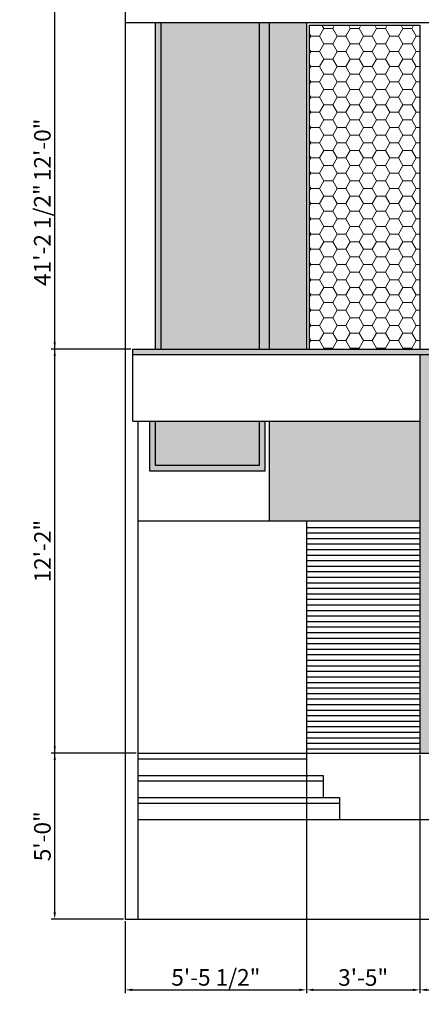
# Model space of a CAD drawing. Units: millimetres. Extents: x 67033 to 68301, y 155969 to 157209.
# Tile 7 of 17: x 67889 to 68034, y 155969 to 156325. Entities that reach past the tile are written whole.
import ezdxf

# ---------------------------------------------------------------- set-up
doc = ezdxf.new("R2010")
doc.units = ezdxf.units.MM
for name, color, linetype, lineweight in [('A-ANNO-DIMS', 2, 'Continuous', 18), ('A-ELEV', 7, 'Continuous', 25), ('A-ELEV-PATT', 252, 'Continuous', 13)]:
    doc.layers.add(name, color=color, linetype=linetype, lineweight=lineweight)
doc.styles.get("Standard").update_dxf_attribs({"font": 'arial.ttf'})
doc.dimstyles.new('ISO-25', dxfattribs={"dimtxt": 6, "dimasz": 2.5, "dimexe": 1.25, "dimexo": 0.625, "dimtad": 1, "dimdec": 0, "dimlunit": 3, "dimtxsty": 'Standard', "dimcen": 2.5, "dimadec": 0, "dimazin": 0, "dimtfac": 1, "dimtdec": 0, "dimtmove": 0, "dimatfit": 3, "dimfxl": 1, "dimarcsym": 0})

# ---------------------------------------------------------------- blocks, each defined once
blk = doc.blocks.new('*D129')
at = {"layer": 'A-ANNO-DIMS', "color": 0, "lineweight": -2, "transparency": 16777216}
for p, q in [((67992.65, 156057.57), (67992.65, 155973.45)), ((67927.19, 155999.57), (67927.19, 155973.45)), ((67929.69, 155974.7), (67990.15, 155974.7))]:
    blk.add_line(p, q, dxfattribs=at)
at = {"layer": 'A-ANNO-DIMS', "color": 0, "transparency": 16777216}
for points in [[(67929.69, 155975.12), (67929.69, 155974.28), (67927.19, 155974.7)], [(67990.15, 155975.12), (67990.15, 155974.28), (67992.65, 155974.7)]]:
    blk.add_solid(points, dxfattribs=at)
at = {"layer": 'Defpoints', "color": 0, "transparency": 16777216}
for p in [(67992.65, 156058.2), (67927.19, 156000.2), (67992.65, 155974.7)]:
    blk.add_point(p, dxfattribs=at)
at = {"layer": 'A-ANNO-DIMS', "color": 0, "transparency": 16777216, "insert": (67959.92, 155978.43), "char_height": 6, "attachment_point": 5}
blk.add_mtext('5\'-5 1/2"', dxfattribs=at)
blk = doc.blocks.new('*D130')
at = {"layer": 'A-ANNO-DIMS', "color": 0, "lineweight": -2, "transparency": 16777216}
for p, q in [((68033.69, 156059.57), (68033.69, 155973.45)), ((67992.65, 156057.57), (67992.65, 155973.45)), ((67995.15, 155974.7), (68031.19, 155974.7))]:
    blk.add_line(p, q, dxfattribs=at)
at = {"layer": 'A-ANNO-DIMS', "color": 0, "transparency": 16777216}
for points in [[(67995.15, 155975.12), (67995.15, 155974.28), (67992.65, 155974.7)], [(68031.19, 155975.12), (68031.19, 155974.28), (68033.69, 155974.7)]]:
    blk.add_solid(points, dxfattribs=at)
at = {"layer": 'Defpoints', "color": 0, "transparency": 16777216}
for p in [(68033.69, 156060.2), (67992.65, 156058.2), (68033.69, 155974.7)]:
    blk.add_point(p, dxfattribs=at)
at = {"layer": 'A-ANNO-DIMS', "color": 0, "transparency": 16777216, "insert": (68013.17, 155978.39), "char_height": 6, "attachment_point": 5}
blk.add_mtext('3\'-5"', dxfattribs=at)
blk = doc.blocks.new('*D131')
at = {"layer": 'A-ANNO-DIMS', "color": 0, "lineweight": -2, "transparency": 16777216}
for p, q in [((68033.69, 156059.57), (68033.69, 155973.45)), ((68057.69, 156059.57), (68057.69, 155973.45)), ((68036.19, 155974.7), (68055.19, 155974.7))]:
    blk.add_line(p, q, dxfattribs=at)
at = {"layer": 'A-ANNO-DIMS', "color": 0, "transparency": 16777216}
for points in [[(68036.19, 155975.12), (68036.19, 155974.28), (68033.69, 155974.7)], [(68055.19, 155975.12), (68055.19, 155974.28), (68057.69, 155974.7)]]:
    blk.add_solid(points, dxfattribs=at)
at = {"layer": 'Defpoints', "color": 0, "transparency": 16777216}
for p in [(68033.69, 156060.2), (68057.69, 156060.2), (68057.69, 155974.7)]:
    blk.add_point(p, dxfattribs=at)
at = {"layer": 'A-ANNO-DIMS', "color": 0, "transparency": 16777216, "insert": (68045.69, 155978.39), "char_height": 6, "attachment_point": 5}
blk.add_mtext('2\'-0"', dxfattribs=at)
blk = doc.blocks.new('*D136')
at = {"layer": 'A-ANNO-DIMS', "color": 0, "lineweight": -2, "transparency": 16777216}
for p, q in [((67931.07, 156060.2), (67900.44, 156060.2)), ((67901.69, 156002.7), (67901.69, 156057.7)), ((67926.57, 156000.2), (67900.44, 156000.2))]:
    blk.add_line(p, q, dxfattribs=at)
at = {"layer": 'A-ANNO-DIMS', "color": 0, "transparency": 16777216}
for points in [[(67901.27, 156057.7), (67902.11, 156057.7), (67901.69, 156060.2)], [(67901.27, 156002.7), (67902.11, 156002.7), (67901.69, 156000.2)]]:
    blk.add_solid(points, dxfattribs=at)
at = {"layer": 'Defpoints', "color": 0, "transparency": 16777216}
for p in [(67901.69, 156060.2), (67931.69, 156060.2), (67927.19, 156000.2)]:
    blk.add_point(p, dxfattribs=at)
at = {"layer": 'A-ANNO-DIMS', "color": 0, "transparency": 16777216, "insert": (67898, 156030.2), "char_height": 6, "attachment_point": 5, "rotation": 90}
blk.add_mtext('5\'-0"', dxfattribs=at)
blk = doc.blocks.new('*D137')
at = {"layer": 'A-ANNO-DIMS', "color": 0, "lineweight": -2, "transparency": 16777216}
for p, q in [((67929.24, 156206.2), (67900.44, 156206.2)), ((67901.69, 156062.7), (67901.69, 156203.7)), ((67931.07, 156060.2), (67900.44, 156060.2))]:
    blk.add_line(p, q, dxfattribs=at)
at = {"layer": 'A-ANNO-DIMS', "color": 0, "transparency": 16777216}
for points in [[(67901.27, 156203.7), (67902.11, 156203.7), (67901.69, 156206.2)], [(67901.27, 156062.7), (67902.11, 156062.7), (67901.69, 156060.2)]]:
    blk.add_solid(points, dxfattribs=at)
at = {"layer": 'Defpoints', "color": 0, "transparency": 16777216}
for p in [(67901.69, 156206.2), (67929.86, 156206.2), (67931.69, 156060.2)]:
    blk.add_point(p, dxfattribs=at)
at = {"layer": 'A-ANNO-DIMS', "color": 0, "transparency": 16777216, "insert": (67898.05, 156133.2), "char_height": 6, "attachment_point": 5, "rotation": 90}
blk.add_mtext('12\'-2"', dxfattribs=at)
blk = doc.blocks.new('*D138')
at = {"layer": 'A-ANNO-DIMS', "color": 0, "lineweight": -2, "transparency": 16777216}
for p, q in [((67926.57, 156350.2), (67900.44, 156350.2)), ((67901.69, 156208.7), (67901.69, 156347.7)), ((67929.24, 156206.2), (67900.44, 156206.2))]:
    blk.add_line(p, q, dxfattribs=at)
at = {"layer": 'A-ANNO-DIMS', "color": 0, "transparency": 16777216}
for points in [[(67901.27, 156347.7), (67902.11, 156347.7), (67901.69, 156350.2)], [(67901.27, 156208.7), (67902.11, 156208.7), (67901.69, 156206.2)]]:
    blk.add_solid(points, dxfattribs=at)
at = {"layer": 'Defpoints', "color": 0, "transparency": 16777216}
for p in [(67901.69, 156350.2), (67927.19, 156350.2), (67929.86, 156206.2)]:
    blk.add_point(p, dxfattribs=at)
at = {"layer": 'A-ANNO-DIMS', "color": 0, "transparency": 16777216, "insert": (67898, 156278.2), "char_height": 6, "attachment_point": 5, "rotation": 90}
blk.add_mtext('12\'-0"', dxfattribs=at)
blk = doc.blocks.new('*D140')
at = {"layer": 'A-ANNO-DIMS', "color": 0, "lineweight": -2, "transparency": 16777216}
for p, q in [((67992.02, 156494.61), (67900.44, 156494.61)), ((67901.69, 156002.7), (67901.69, 156492.11)), ((67926.57, 156000.2), (67900.44, 156000.2))]:
    blk.add_line(p, q, dxfattribs=at)
at = {"layer": 'A-ANNO-DIMS', "color": 0, "transparency": 16777216}
for points in [[(67901.27, 156492.11), (67902.11, 156492.11), (67901.69, 156494.61)], [(67901.27, 156002.7), (67902.11, 156002.7), (67901.69, 156000.2)]]:
    blk.add_solid(points, dxfattribs=at)
at = {"layer": 'Defpoints', "color": 0, "transparency": 16777216}
for p in [(67901.69, 156494.61), (67992.65, 156494.61), (67927.19, 156000.2)]:
    blk.add_point(p, dxfattribs=at)
at = {"layer": 'A-ANNO-DIMS', "color": 0, "transparency": 16777216, "insert": (67897.96, 156247.4), "char_height": 6, "attachment_point": 5, "rotation": 90}
blk.add_mtext('41\'-2 1/2"', dxfattribs=at)

msp = doc.modelspace()

# ---------------------------------------------------------------- hatches: boundary and pattern name
at = {"layer": 'A-ELEV-PATT'}
h = msp.add_hatch(color=256, dxfattribs=at)
h.dxf.hatch_style = 1
h.paths.add_polyline_path([(67940.11, 156324.2), (67938.11, 156324.2), (67938.11, 156206.2), (67940.11, 156206.2)])
h = msp.add_hatch(color=256, dxfattribs=at)
h.dxf.hatch_style = 1
h.paths.add_polyline_path([(67975.63, 156324.2), (67940.11, 156324.2), (67940.11, 156206.2), (67975.63, 156206.2)])
h = msp.add_hatch(color=256, dxfattribs=at)
h.dxf.hatch_style = 1
h.paths.add_polyline_path([(67979.14, 156324.2), (67975.63, 156324.2), (67975.63, 156206.2), (67979.14, 156206.2)])
h = msp.add_hatch(color=256, dxfattribs=at)
h.dxf.hatch_style = 1
h.paths.add_polyline_path([(67992.65, 156324.2), (67979.14, 156324.2), (67979.14, 156206.2), (67992.65, 156206.2)])
h = msp.add_hatch(dxfattribs=at)
h.set_pattern_fill('HONEY', color=256)
h.paths.add_polyline_path([(68033.69, 156323.2), (67993.65, 156323.2), (67993.65, 156206.2), (68033.69, 156206.2)])
h = msp.add_hatch(color=256, dxfattribs=at)
h.dxf.hatch_style = 1
h.paths.add_polyline_path([(68166.64, 156206.2), (67929.86, 156206.2), (67929.86, 156204.2), (68166.64, 156204.2)])
h = msp.add_hatch(color=256, dxfattribs=at)
h.dxf.hatch_style = 1
h.paths.add_polyline_path([(68175.64, 156180.2), (68092.61, 156180.2), (68092.61, 156197.05), (68166.64, 156197.05), (68166.64, 156204.2), (68033.69, 156204.2), (68033.69, 156060.2), (68039.69, 156060.2), (68039.69, 156160.28), (68051.69, 156160.28), (68051.69, 156060.2), (68057.69, 156060.2), (68057.69, 156160.28), (68133.69, 156160.28), (68165.64, 156160.28), (68165.64, 156060.2), (68175.64, 156060.2)])
h = msp.add_hatch(color=256, dxfattribs=at)
h.dxf.hatch_style = 1
h.paths.add_polyline_path([(67977.63, 156180.2), (67975.63, 156180.2), (67975.63, 156164.15), (67938.11, 156164.15), (67938.11, 156180.2), (67936.11, 156180.2), (67936.11, 156162.15), (67977.63, 156162.15)])
h = msp.add_hatch(color=256, dxfattribs=at)
h.dxf.hatch_style = 1
h.paths.add_polyline_path([(67975.63, 156180.2), (67938.11, 156180.2), (67938.11, 156164.15), (67975.63, 156164.15)])
h = msp.add_hatch(color=256, dxfattribs=at)
h.dxf.hatch_style = 1
h.paths.add_polyline_path([(68033.69, 156180.2), (67979.14, 156180.2), (67979.14, 156144.2), (68033.69, 156144.2)])

# ---------------------------------------------------------------- linework, layer by layer
at = {"layer": 'A-ELEV'}
for p, q in [((67927.19, 156486.2), (67927.19, 156000.2)), ((67927.19, 156324.2), (68166.64, 156324.2)), ((67938.11, 156206.2), (67938.11, 156324.2)), ((67940.11, 156206.2), (67940.11, 156324.2)), ((67975.63, 156324.2), (67975.63, 156206.2)), ((67979.14, 156324.2), (67979.14, 156206.2)), ((67992.65, 156324.2), (67992.65, 156206.2)), ((67993.65, 156323.2), (67993.65, 156206.2)), ((67993.65, 156323.2), (68033.69, 156323.2)), ((68033.69, 156323.2), (68033.69, 156206.2)), ((67929.86, 156206.2), (68166.64, 156206.2)), ((67929.86, 156180.2), (67929.86, 156206.2)), ((67929.86, 156204.2), (68166.64, 156204.2)), ((68033.69, 156204.2), (68033.69, 156060.2)), ((67929.86, 156180.2), (68033.69, 156180.2)), ((67931.69, 156180.2), (67931.69, 156000.2)), ((67938.11, 156164.15), (67938.11, 156180.2)), ((67975.63, 156180.2), (67975.63, 156164.15)), ((67979.14, 156180.2), (67979.14, 156144.2)), ((67975.63, 156164.15), (67938.11, 156164.15)), ((67931.69, 156144.2), (68033.69, 156144.2)), ((67992.65, 156144.2), (67992.65, 156052.2)), ((67992.65, 156141.81), (68033.69, 156141.81)), ((67992.65, 156139.81), (68033.69, 156139.81)), ((67992.65, 156137.81), (68033.69, 156137.81)), ((67992.65, 156135.81), (68033.69, 156135.81)), ((67992.65, 156133.81), (68033.69, 156133.81)), ((67992.65, 156131.81), (68033.69, 156131.81)), ((67992.65, 156129.81), (68033.69, 156129.81)), ((67992.65, 156127.81), (68033.69, 156127.81)), ((67992.65, 156125.81), (68033.69, 156125.81)), ((67992.65, 156123.81), (68033.69, 156123.81)), ((67992.65, 156121.81), (68033.69, 156121.81)), ((67992.65, 156119.81), (68033.69, 156119.81)), ((67992.65, 156117.81), (68033.69, 156117.81)), ((67992.65, 156115.81), (68033.69, 156115.81)), ((67992.65, 156113.81), (68033.69, 156113.81)), ((67992.65, 156111.81), (68033.69, 156111.81)), ((67992.65, 156109.81), (68033.69, 156109.81)), ((67992.65, 156107.81), (68033.69, 156107.81)), ((67992.65, 156105.81), (68033.69, 156105.81)), ((67992.65, 156103.81), (68033.69, 156103.81)), ((67992.65, 156101.81), (68033.69, 156101.81)), ((67992.65, 156099.81), (68033.69, 156099.81)), ((67992.65, 156097.81), (68033.69, 156097.81)), ((67992.65, 156095.81), (68033.69, 156095.81)), ((67992.65, 156093.81), (68033.69, 156093.81)), ((67992.65, 156091.81), (68033.69, 156091.81)), ((67992.65, 156089.81), (68033.69, 156089.81)), ((67992.65, 156087.81), (68033.69, 156087.81)), ((67992.65, 156085.81), (68033.69, 156085.81)), ((67992.65, 156083.81), (68033.69, 156083.81)), ((67992.65, 156081.81), (68033.69, 156081.81)), ((67992.65, 156079.81), (68033.69, 156079.81)), ((67992.65, 156077.81), (68033.69, 156077.81)), ((67992.65, 156075.81), (68033.69, 156075.81)), ((67992.65, 156073.81), (68033.69, 156073.81)), ((67992.65, 156071.81), (68033.69, 156071.81)), ((67992.65, 156069.81), (68033.69, 156069.81)), ((67992.65, 156067.81), (68033.69, 156067.81)), ((67992.65, 156065.81), (68033.69, 156065.81)), ((67992.65, 156063.81), (68033.69, 156063.81)), ((67931.69, 156060.2), (68266.19, 156060.2)), ((67992.65, 156061.81), (68033.69, 156061.81)), ((67931.69, 156058.2), (67992.65, 156058.2)), ((67931.69, 156052.2), (67992.65, 156052.2)), ((67992.65, 156052.2), (67998.66, 156052.2)), ((67998.66, 156052.2), (67998.66, 156044.2)), ((67931.69, 156050.2), (67998.66, 156050.2)), ((67931.69, 156044.2), (67998.66, 156044.2)), ((67998.66, 156044.2), (68004.58, 156044.2)), ((68004.58, 156044.2), (68004.58, 156036.2)), ((67931.69, 156042.2), (68004.58, 156042.2)), ((67931.69, 156036.2), (68004.58, 156036.2)), ((68004.58, 156036.2), (68194.31, 156036.2)), ((67927.19, 156000.2), (68266.19, 156000.2))]:
    msp.add_line(p, q, dxfattribs=at)
msp.add_lwpolyline([(67936.11, 156180.2), (67977.63, 156180.2), (67977.63, 156162.15), (67936.11, 156162.15)], close=True, dxfattribs=at)

# ---------------------------------------------------------------- dimensions: what is measured, and where the dimension line sits
at = {"layer": 'A-ANNO-DIMS'}
for base, p1, p2, picture, middle in [((67901.69, 156494.61), (67927.19, 156000.2), (67992.65, 156494.61), '*D140', (67897.96, 156247.4)), ((67901.69, 156350.2), (67929.86, 156206.2), (67927.19, 156350.2), '*D138', (67898, 156278.2)), ((67901.69, 156206.2), (67931.69, 156060.2), (67929.86, 156206.2), '*D137', (67898.05, 156133.2)), ((67901.69, 156060.2), (67927.19, 156000.2), (67931.69, 156060.2), '*D136', (67898, 156030.2))]:
    dim = msp.add_linear_dim(base=base, p1=p1, p2=p2, angle=90, dimstyle='ISO-25', override={"dimdec": 1, "dimlfac": 1, "dimrnd": 0, "dimzin": 1, "dimdsep": 46, "dimlunit": 4, "dimfrac": 2}, dxfattribs=at)
    dim.commit()
    dim.dimension.update_dxf_attribs({"geometry": picture, "text_midpoint": middle})
for base, p1, p2, picture, middle in [((68033.69, 155974.7), (67992.65, 156058.2), (68033.69, 156060.2), '*D130', (68013.17, 155978.39)), ((68057.69, 155974.7), (68033.69, 156060.2), (68057.69, 156060.2), '*D131', (68045.69, 155978.39)), ((67992.65, 155974.7), (67927.19, 156000.2), (67992.65, 156058.2), '*D129', (67959.92, 155978.43))]:
    dim = msp.add_linear_dim(base=base, p1=p1, p2=p2, dimstyle='ISO-25', override={"dimdec": 1, "dimlfac": 1, "dimrnd": 0, "dimzin": 1, "dimdsep": 46, "dimlunit": 4, "dimfrac": 2}, dxfattribs=at)
    dim.commit()
    dim.dimension.update_dxf_attribs({"geometry": picture, "text_midpoint": middle})

doc.saveas('drawing.dxf')
